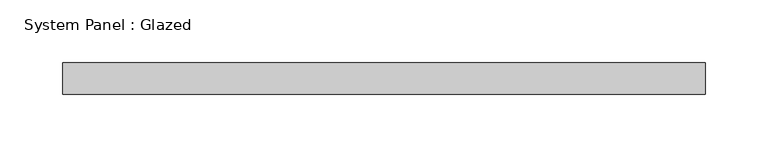
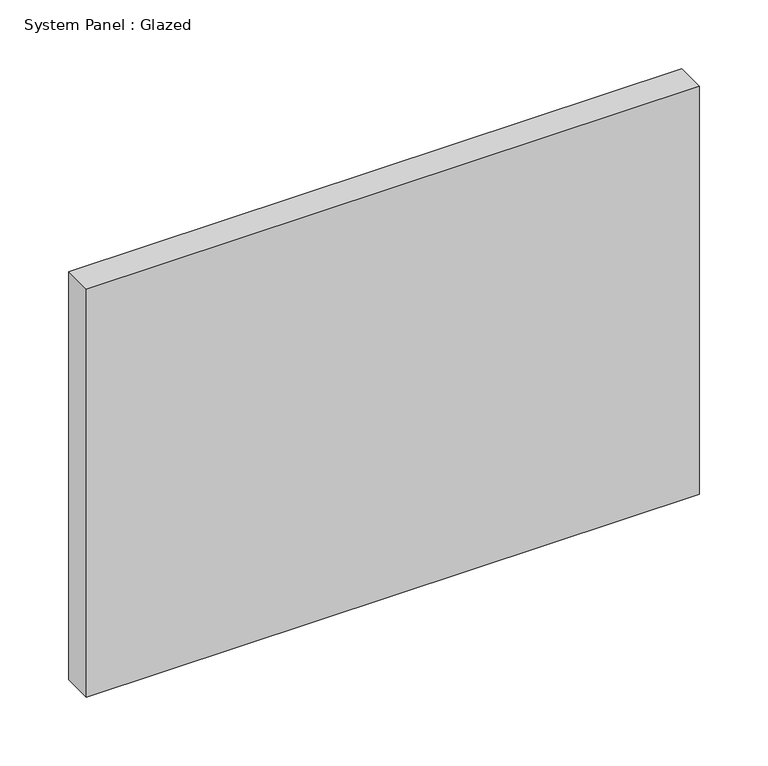
"""IFC4 building model written with IfcOpenShell, lengths in millimetres: plate geometry, System Panel : Glazed."""

from ifc_helpers import new_model, si_unit, origin, origin_with_axes, place, context, project, spatial, polyline, outline, extrude, source, transform, mapped, element, save


def system_panel_glazed_6374c067(model_context):
    return source(origin(), model_context, "Body", "SweptSolid", [
        extrude(outline(polyline([(257.175, 19.05), (-257.175, 19.05), (-257.175, 44.45), (257.175, 44.45), (257.175, 19.05)])), origin_with_axes(), (0.0, 0.0, 1.0), 361.95),
    ])


if __name__ == "__main__":
    model = new_model("IFC4")
    model_context = context("Model", 3, world=origin())
    ifc_project = project(units=[si_unit("LENGTHUNIT", "METRE", prefix="MILLI")], contexts=[model_context])
    site = spatial("IfcSite", under=ifc_project)
    building = spatial("IfcBuilding", under=site)
    placement = place(None, origin())
    system_panel_glazed_shape = system_panel_glazed_6374c067(model_context)
    element("IfcPlate", 1, ObjectType="System Panel : Glazed", at=placement, inside=building, context=model_context, shape_type="MappedRepresentation", body=[
        mapped(system_panel_glazed_shape, transform((0.0, 0.0, 0.0), x_axis=(1.0, 0.0, 0.0), y_axis=(0.0, 1.0, 0.0), z_axis=(0.0, 0.0, 1.0))),
    ])
    save(model, "model.ifc")

# Revit data of these elements
# Type "System Panel : Glazed"
#   Construction Type Id = "GSP4R"
#   Analytic Construction = "1/8 in Pilkington single glazing"
#   Visual Light Transmittance = 0.9
#   Solar Heat Gain Coefficient = 0.86
#   Heat Transfer Coefficient (U) = 1.18115 BTU/(h·ft²·°F)
#   Define Thermal Properties by = 1
# Element 1 (IfcPlate, "System Panel : Glazed")
#   Materials on its faces: "Glass"
# Materials
#   "Glass": class "Glass", colour RGB 0 128 192, transparency 0.75, Description = "Soda Lime Glass", Cost = 0
